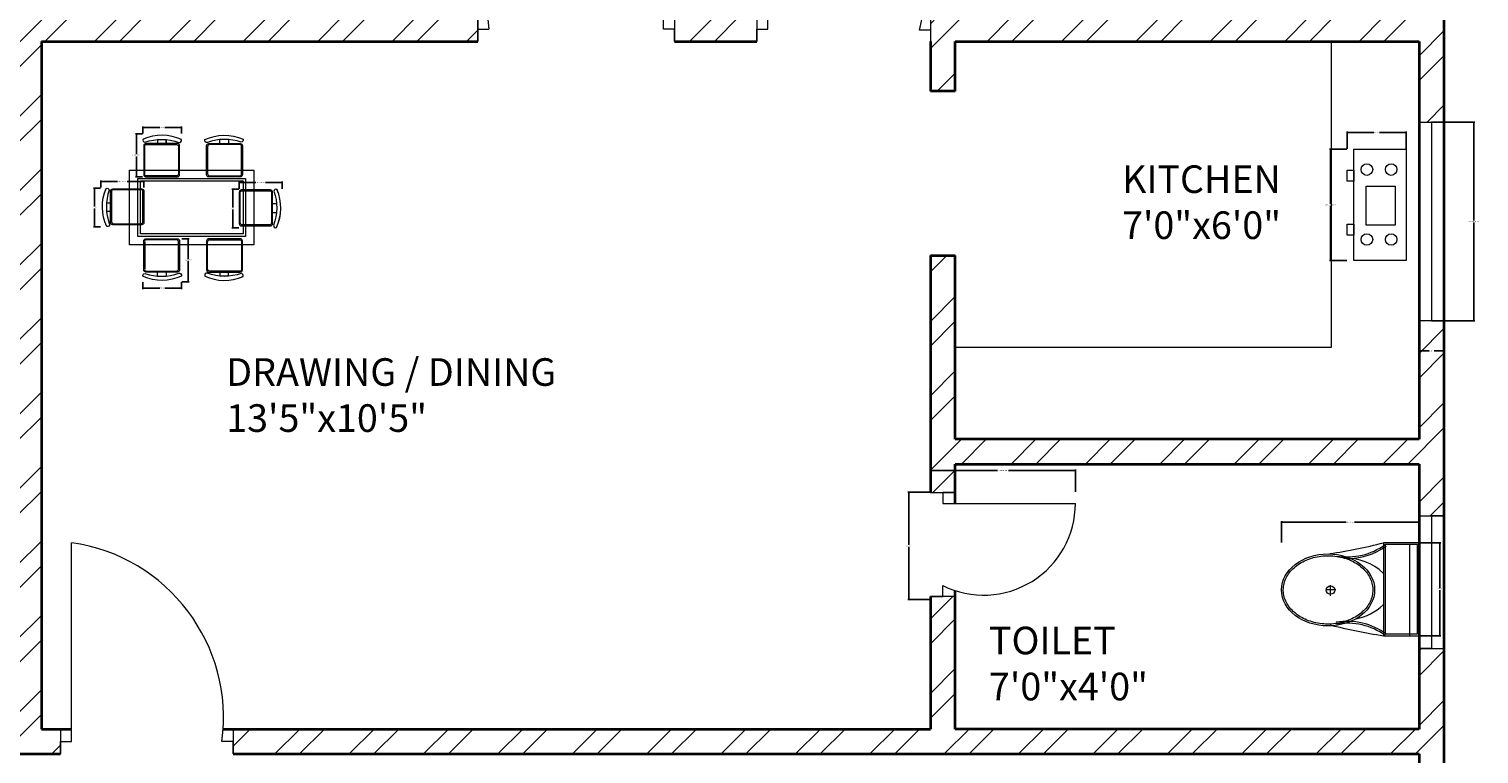
# Model space of a CAD drawing. Units: inches. Extents: x 1944 to 3454, y 1352 to 3055.
# Tile 8 of 17: x 2314 to 2576, y 1900 to 2031. Entities that reach past the tile are written whole.
import ezdxf

# ---------------------------------------------------------------- set-up
doc = ezdxf.new("R2010")
doc.units = ezdxf.units.IN
for name, color, linetype, lineweight in [('A-ANNO-DIMS', 2, 'Continuous', 18), ('A-AREA-IDEN', 7, 'Continuous', 18), ('A-DOOR', 3, 'Continuous', 20), ('A-EQPM', 9, 'Continuous', 18), ('A-FLOR-CASE', 8, 'Continuous', 20), ('A-FLOR-FIXT', 9, 'Continuous', 18), ('A-FURN', 8, 'Continuous', 13), ('A-GLAZ', 4, 'Continuous', 18), ('A-WALL', 7, 'Continuous', 35), ('A-WALL-PATT', 252, 'Continuous', 13)]:
    doc.layers.add(name, color=color, linetype=linetype, lineweight=lineweight)
doc.styles.get("Standard").update_dxf_attribs({"font": 'arial.ttf'})
doc.dimstyles.get("Standard").update_dxf_attribs({"dimtxt": 0.18, "dimasz": 0.18, "dimexe": 0.18, "dimexo": 0.0625, "dimgap": 0.09, "dimtad": 0, "dimtih": 1, "dimtoh": 1, "dimdec": 4, "dimzin": 0, "dimdsep": 46, "dimtxsty": 'Standard', "dimcen": 0.09, "dimadec": 0, "dimazin": 0, "dimtfac": 1, "dimtdec": 4, "dimtofl": 0, "dimtmove": 0, "dimatfit": 3, "dimfxl": 1, "dimtolj": 1, "dimtzin": 0, "dimarcsym": 0})

# ---------------------------------------------------------------- blocks, each defined once
blk = doc.blocks.new('A$C31115884')
for p, q in [((283.1, 497.7), (223.4, 497.7)), ((257.5, 466.4), (257.5, 523.2)), ((0, 200), (0, 0)), ((520, 200), (0, 200)), ((10, 190), (10, 10)), ((510, 190), (10, 190)), ((510, 10), (510, 190)), ((520, 0), (520, 200)), ((510, 54.5), (0, 54.5)), ((10, 10), (510, 10)), ((0, 0), (520, 0))]:
    blk.add_line(p, q)
blk.add_circle((255.6, 496.4), 23.6)
for centre, radius, start, end in [((2777.7, -204.6), 2807, 165.4549, 171.71327), ((3237, 905), 2807, 188.28673, 194.5451), ((-294.5, 403.3), 364.7, 324.20913, 9.34987), ((-294.5, 403.3), 374.7, 324.20913, 9.34987), ((139.5, 406.2), 293.5, 315.84364, 2.65635), ((805.8, 403.3), 374.7, 179.20365, 215.79087), ((805.8, 403.3), 364.7, 170.65013, 215.79087), ((383.6, 406.2), 293.5, 190.27735, 224.15636)]:
    blk.add_arc(centre, radius, start, end)
blk.add_ellipse((256.2, 509.9), major_axis=(0, -260.7), ratio=0.772727)
blk.add_open_spline([(256.2, 259.2), (263.1, 259.2), (270, 259.7), (287.8, 262.3), (298.7, 265.1), (319.9, 273.1), (330.2, 278.4), (350.1, 291.1), (359.7, 298.7), (377.7, 315.9), (386.2, 325.5), (401.7, 346.6), (408.8, 358.1), (421.3, 382.5), (426.8, 395.5), (435.9, 422.4), (439.5, 436.4), (444.8, 465.1), (446.5, 479.7), (447.9, 509.2), (447.6, 524), (445, 553.3), (442.7, 567.8), (436.3, 596), (432.1, 609.7), (421.9, 636), (416, 648.6), (402.5, 672.1), (395, 683), (378.6, 703), (369.8, 712.1), (351.1, 728), (341.3, 734.8), (320.9, 746.2), (310.4, 750.7), (288.9, 757.3), (278, 759.4), (256, 761), (245, 760.6), (223.1, 757.2), (212.3, 754.3), (191.1, 746.1), (180.8, 740.7), (160.9, 727.8), (151.4, 720.1), (133.5, 702.7), (125.1, 693), (109.6, 671.7), (102.6, 660.2), (90.2, 635.7), (84.9, 622.7), (76, 595.6), (72.4, 581.6), (67.2, 552.9), (65.6, 538.2), (64.4, 508.8), (64.8, 494), (67.5, 464.7), (69.9, 450.2), (76.6, 422), (80.8, 408.3), (91.1, 382.2), (97.2, 369.7), (110.8, 346.3), (118.4, 335.4), (134.8, 315.6), (143.7, 306.7), (162.4, 290.9), (172.3, 284.2), (192.8, 273), (203.3, 268.6), (224.8, 262.2), (235.8, 260.2), (249.9, 259.3), (253, 259.2), (256.2, 259.2)], degree=3, knots=[0, 0, 0, 0, 0.110105, 0.110105, 0.285049, 0.285049, 0.459994, 0.459994, 0.634938, 0.634938, 0.809882, 0.809882, 0.984827, 0.984827, 1.159771, 1.159771, 1.334715, 1.334715, 1.50966, 1.50966, 1.684604, 1.684604, 1.859549, 1.859549, 2.034493, 2.034493, 2.209437, 2.209437, 2.384382, 2.384382, 2.559326, 2.559326, 2.73427, 2.73427, 2.909215, 2.909215, 3.084159, 3.084159, 3.259103, 3.259103, 3.434048, 3.434048, 3.608992, 3.608992, 3.783936, 3.783936, 3.958881, 3.958881, 4.133825, 4.133825, 4.30877, 4.30877, 4.483714, 4.483714, 4.658658, 4.658658, 4.833603, 4.833603, 5.008547, 5.008547, 5.183491, 5.183491, 5.358436, 5.358436, 5.53338, 5.53338, 5.708324, 5.708324, 5.883269, 5.883269, 6.058213, 6.058213, 6.233158, 6.233158, 6.283185, 6.283185, 6.283185, 6.283185])
blk = doc.blocks.new('COOKTOP-4B-01')
for points in [[(0, 20.18), (9.48, 20.18), (9.48, 0), (0, 0)], [(2, 13.79), (7.26, 13.79), (7.26, 6.73), (2, 6.73)], [(9.48, 15.59), (10.71, 15.59), (10.71, 13.59), (9.48, 13.59)], [(9.48, 5.81), (10.71, 5.81), (10.71, 3.8), (9.48, 3.8)]]:
    blk.add_lwpolyline(points, close=True)
for centre in [(2.74, 16.38), (7.14, 16.38), (2.74, 3.71), (7.14, 3.71)]:
    blk.add_circle(centre, 1.05)
blk = doc.blocks.new('DOOR-SWING-36IN-01')
for p, q in [((33.61, 2.25), (33.61, 38.25)), ((0, 4.5), (0, 0)), ((0, 0), (0, 4.5)), ((0, 4.5), (0, 2.25)), ((35.61, 4.5), (35.61, 0)), ((0, 2.25), (2, 2.25)), ((35.61, 2.25), (33.61, 2.25)), ((35.61, 0), (35.61, 2.25))]:
    blk.add_line(p, q)
blk.add_arc((33.61, 6.37), 31.88, 90, 187.4328)
blk = doc.blocks.new('DOOR-SWING-36IN-02')
for p, q in [((2, 2.65), (2, 38.65)), ((0, 4.9), (0, 0.4)), ((0, 0.4), (0, 2.65)), ((0, 2.65), (2, 2.65)), ((31.45, 4.9), (31.45, 0)), ((31.45, 2.45), (29.45, 2.45))]:
    blk.add_line(p, q)
blk.add_arc((2, 10.14), 28.51, 344.3464, 90)
blk = doc.blocks.new('DOOR-SWING-24IN-05')
for p, q in [((0, 18.87), (4.5, 18.87)), ((4.5, 18.87), (2.25, 18.87)), ((2.25, 18.87), (2.25, 16.87)), ((2.25, 16.87), (26.25, 16.87)), ((4.5, 0), (0, 0)), ((0, 0), (2.25, 0)), ((2.25, 0), (2.25, 2))]:
    blk.add_line(p, q)
blk.add_arc((9.64, 16.87), 16.61, 243.5781, 0)
blk = doc.blocks.new('DOOR-SWING-36IN-09')
for p, q in [((2, 2.25), (2, 38.25)), ((0, 4.5), (0, 0)), ((31.24, 4.5), (31.24, 0)), ((0, 0), (0, 2.25)), ((0, 2.25), (2, 2.25)), ((31.24, 2.25), (29.24, 2.25)), ((31.24, 0), (31.24, 2.25))]:
    blk.add_line(p, q)
blk.add_arc((-2.49, 6.55), 32.02, 352.2825, 81.9468)
blk = doc.blocks.new('WINDOW-PLAN-24.00IN-01')
for p, q in [((2.25, 24), (0, 24)), ((0, 24), (4.5, 24)), ((2.25, 0), (2.25, 24)), ((0, 0), (4.5, 0)), ((4.5, 0), (2.25, 0))]:
    blk.add_line(p, q)
blk = doc.blocks.new('WINDOW-PLAN-36.00IN-02')
for p, q in [((0, 36), (4.5, 36)), ((4.5, 36), (2.25, 36)), ((2.25, 36), (2.25, 0)), ((4.5, 0), (0, 0)), ((2.25, 0), (4.5, 0))]:
    blk.add_line(p, q)
blk = doc.blocks.new('TABLE-DINING-01')
for points in [[(0, 13.51), (22.52, 13.51), (22.52, 0), (0, 0)], [(0, 13.51), (22.52, 13.51), (22.52, 0), (0, 0)], [(1.5, 12.01), (21.02, 12.01), (21.02, 1.5), (1.5, 1.5)], [(1.5, 12.01), (21.02, 12.01), (21.02, 1.5), (1.5, 1.5)], [(1.95, 11.56), (20.57, 11.56), (20.57, 1.95), (1.95, 1.95)], [(1.95, 11.56), (20.57, 11.56), (20.57, 1.95), (1.95, 1.95)]]:
    blk.add_lwpolyline(points, close=True)
blk = doc.blocks.new('CHAIR-DINING-03')
for points in [[(6.03, 6.44, 0.414214), (5.63, 6.84), (0.4, 6.84, 0.414214), (0, 6.44), (0, 0.74, 0.414214), (0.4, 0.35), (5.63, 0.35, 0.414214), (6.03, 0.74), (6.03, 6.44)], [(6.28, 6.62, -0.175809), (6.23, 0.48, 0.578392), (6.74, 0.02, 0.214524), (6.84, 6.94, 0.552014), (6.28, 6.62, -0.065079)], [(6.03, 2.74), (6.75, 2.74, -0.064759)]]:
    blk.add_lwpolyline(points, format="xyb")
blk.add_lwpolyline([(5.85, 6.44), (5.85, 0.92, -0.414214), (5.45, 0.52), (0.58, 0.52, -0.414214), (0.18, 0.92), (0.18, 6.44, -0.512069), (0.58, 6.66), (5.45, 6.66, -0.512069)], format="xyb", close=True)
blk.add_lwpolyline([(6.77, 4.34), (6.03, 4.34)])
blk = doc.blocks.new('CHAIR-DINING-05')
for points in [[(6.44, 1.5, 0.414214), (6.84, 1.9), (6.84, 7.13, 0.414214), (6.44, 7.53), (0.74, 7.53, 0.414214), (0.34, 7.13), (0.34, 1.9, 0.414214), (0.74, 1.5), (6.44, 1.5)], [(6.62, 1.25, -0.175809), (0.48, 1.3, 0.578392), (0.02, 0.79, 0.214524), (6.94, 0.7, 0.552014), (6.62, 1.25, -0.065079)], [(2.74, 1.5), (2.74, 0.78, -0.064759)]]:
    blk.add_lwpolyline(points, format="xyb")
blk.add_lwpolyline([(6.44, 1.68), (0.92, 1.68, -0.414214), (0.52, 2.08), (0.52, 6.95, -0.414214), (0.92, 7.35), (6.44, 7.35, -0.512069), (6.66, 6.95), (6.66, 2.08, -0.512069)], format="xyb", close=True)
blk.add_lwpolyline([(4.34, 0.77), (4.34, 1.5)])
blk = doc.blocks.new('CHAIR-DINING-06')
for points in [[(0.37, 6.28, -0.175809), (6.5, 6.23, 0.578392), (6.97, 6.74, 0.214524), (0.04, 6.84, 0.552014), (0.37, 6.28, -0.065079)], [(6.24, 6.03), (0.55, 6.03, 0.414214), (0.15, 5.63), (0.15, 0.4, 0.414214), (0.55, 0), (6.24, 0, 0.414214), (6.64, 0.4), (6.64, 5.63, 0.414214), (6.24, 6.03)], [(4.24, 6.03), (4.24, 6.75, -0.064759)]]:
    blk.add_lwpolyline(points, format="xyb")
blk.add_lwpolyline([(0.55, 5.85), (6.06, 5.85, -0.414214), (6.46, 5.46), (6.46, 0.58, -0.414214), (6.06, 0.18), (0.55, 0.18, -0.512069), (0.33, 0.58), (0.33, 5.46, -0.512069)], format="xyb", close=True)
blk.add_lwpolyline([(2.65, 6.77), (2.65, 6.03)])
blk = doc.blocks.new('CHAIR-DINING-07')
for points in [[(1.3, 0.48, -0.578392), (0.79, 0.02, -0.214524), (0.7, 6.94, -0.552014), (1.25, 6.62, 0.175809), (1.3, 0.48)], [(1.5, 6.44, -0.414214), (1.9, 6.84), (7.13, 6.84, -0.414214), (7.53, 6.44), (7.53, 0.74, -0.414214), (7.13, 0.34), (1.9, 0.34, -0.414214), (1.5, 0.74), (1.5, 6.44)], [(1.5, 2.74), (0.78, 2.74, 0.064759)]]:
    blk.add_lwpolyline(points, format="xyb")
blk.add_lwpolyline([(1.68, 6.44), (1.68, 0.92, 0.414214), (2.08, 0.52), (6.95, 0.52, 0.414214), (7.35, 0.92), (7.35, 6.44, 0.512069), (6.95, 6.66), (2.08, 6.66, 0.512069)], format="xyb", close=True)
blk.add_lwpolyline([(0.77, 4.34), (1.5, 4.34)])
blk = doc.blocks.new('CHAIR-DINING-08')
for points in [[(1.3, 0.48, -0.578392), (0.79, 0.02, -0.214524), (0.7, 6.94, -0.552014), (1.25, 6.62, 0.175809), (1.3, 0.48)], [(1.5, 6.44, -0.414214), (1.9, 6.84), (7.13, 6.84, -0.414214), (7.53, 6.44), (7.53, 0.74, -0.414214), (7.13, 0.35), (1.9, 0.35, -0.414214), (1.5, 0.74), (1.5, 6.44)], [(1.5, 2.74), (0.78, 2.74, 0.064759)]]:
    blk.add_lwpolyline(points, format="xyb")
blk.add_lwpolyline([(1.68, 6.44), (1.68, 0.92, 0.414214), (2.08, 0.52), (6.95, 0.52, 0.414214), (7.35, 0.92), (7.35, 6.44, 0.512069), (6.95, 6.66), (2.08, 6.66, 0.512069)], format="xyb", close=True)
blk.add_lwpolyline([(0.77, 4.34), (1.5, 4.34)])
blk = doc.blocks.new('CHAIR-DINING-09')
for points in [[(6.24, 1.5), (0.55, 1.5, -0.414214), (0.15, 1.9), (0.15, 7.13, -0.414214), (0.55, 7.53), (6.24, 7.53, -0.414214), (6.64, 7.13), (6.64, 1.9, -0.414214), (6.24, 1.5)], [(6.5, 1.3, -0.578392), (6.97, 0.79, -0.214524), (0.04, 0.7, -0.552014), (0.37, 1.25, 0.175809), (6.5, 1.3)], [(4.24, 1.5), (4.24, 0.78, 0.064759)]]:
    blk.add_lwpolyline(points, format="xyb")
blk.add_lwpolyline([(0.55, 1.68), (6.06, 1.68, 0.414214), (6.46, 2.08), (6.46, 6.95, 0.414214), (6.06, 7.35), (0.55, 7.35, 0.512069), (0.33, 6.95), (0.33, 2.08, 0.512069)], format="xyb", close=True)
blk.add_lwpolyline([(2.65, 0.77), (2.65, 1.5)])
blk = doc.blocks.new('*D66')
at = {"layer": 'A-ANNO-DIMS', "color": 0, "lineweight": -2, "transparency": 16777216}
for p, q in [((2540.4, 1938.4), (2540.4, 1942.25)), ((2540.58, 1942.07), (2552.08, 1942.07)), ((2565.14, 1942.07), (2553.64, 1942.07)), ((2565.32, 1938.4), (2565.32, 1942.25))]:
    blk.add_line(p, q, dxfattribs=at)
at = {"layer": 'A-ANNO-DIMS', "color": 0, "transparency": 16777216}
for points in [[(2540.58, 1942.1), (2540.58, 1942.04), (2540.4, 1942.07)], [(2565.14, 1942.1), (2565.14, 1942.04), (2565.32, 1942.07)]]:
    blk.add_solid(points, dxfattribs=at)
at = {"layer": 'Defpoints', "color": 0, "transparency": 16777216}
for p in [(2540.4, 1942.07), (2540.4, 1938.33), (2565.32, 1938.33)]:
    blk.add_point(p, dxfattribs=at)
at = {"layer": 'A-ANNO-DIMS', "color": 0, "transparency": 16777216, "insert": (2552.86, 1942.07), "char_height": 0.18, "attachment_point": 5}
blk.add_mtext('\\A1;WC 25 TYP.', dxfattribs=at)
blk = doc.blocks.new('*D67')
at = {"layer": 'A-ANNO-DIMS', "color": 0, "lineweight": -2, "transparency": 16777216}
for p, q in [((2565.38, 1938.33), (2569.24, 1938.33)), ((2569.06, 1938.15), (2569.06, 1930.1)), ((2569.06, 1921.69), (2569.06, 1929.74)), ((2565.38, 1921.51), (2569.24, 1921.51))]:
    blk.add_line(p, q, dxfattribs=at)
at = {"layer": 'A-ANNO-DIMS', "color": 0, "transparency": 16777216}
for points in [[(2569.03, 1938.15), (2569.09, 1938.15), (2569.06, 1938.33)], [(2569.03, 1921.69), (2569.09, 1921.69), (2569.06, 1921.51)]]:
    blk.add_solid(points, dxfattribs=at)
at = {"layer": 'Defpoints', "color": 0, "transparency": 16777216}
for p in [(2565.32, 1938.33), (2569.06, 1938.33), (2565.32, 1921.51)]:
    blk.add_point(p, dxfattribs=at)
at = {"layer": 'A-ANNO-DIMS', "color": 0, "transparency": 16777216, "insert": (2569.06, 1929.92), "char_height": 0.18, "attachment_point": 5}
blk.add_mtext('\\A1;17 TYP.', dxfattribs=at)
blk = doc.blocks.new('*D68')
at = {"layer": 'A-ANNO-DIMS', "color": 0, "lineweight": -2, "transparency": 16777216}
for p, q in [((2552.23, 2009.61), (2549.09, 2009.61)), ((2549.27, 2009.43), (2549.27, 1999.71)), ((2549.27, 1989.62), (2549.27, 1999.34)), ((2552.23, 1989.44), (2549.09, 1989.44))]:
    blk.add_line(p, q, dxfattribs=at)
at = {"layer": 'A-ANNO-DIMS', "color": 0, "transparency": 16777216}
for points in [[(2549.24, 2009.43), (2549.3, 2009.43), (2549.27, 2009.61)], [(2549.24, 1989.62), (2549.3, 1989.62), (2549.27, 1989.44)]]:
    blk.add_solid(points, dxfattribs=at)
at = {"layer": 'Defpoints', "color": 0, "transparency": 16777216}
for p in [(2552.29, 2009.61), (2549.27, 1989.44), (2552.29, 1989.44)]:
    blk.add_point(p, dxfattribs=at)
at = {"layer": 'A-ANNO-DIMS', "color": 0, "transparency": 16777216, "insert": (2549.27, 1999.53), "char_height": 0.18, "attachment_point": 5}
blk.add_mtext('\\A1;COOKTOP 20 TYP.', dxfattribs=at)
blk = doc.blocks.new('*D69')
at = {"layer": 'A-ANNO-DIMS', "color": 0, "lineweight": -2, "transparency": 16777216}
for p, q in [((2552.29, 2009.68), (2552.29, 2012.82)), ((2552.47, 2012.64), (2557.13, 2012.64)), ((2562.82, 2012.64), (2558.17, 2012.64)), ((2563, 2009.68), (2563, 2012.82))]:
    blk.add_line(p, q, dxfattribs=at)
at = {"layer": 'A-ANNO-DIMS', "color": 0, "transparency": 16777216}
for points in [[(2552.47, 2012.67), (2552.47, 2012.61), (2552.29, 2012.64)], [(2562.82, 2012.67), (2562.82, 2012.61), (2563, 2012.64)]]:
    blk.add_solid(points, dxfattribs=at)
at = {"layer": 'Defpoints', "color": 0, "transparency": 16777216}
for p in [(2552.29, 2012.64), (2552.29, 2009.61), (2563, 2009.61)]:
    blk.add_point(p, dxfattribs=at)
at = {"layer": 'A-ANNO-DIMS', "color": 0, "transparency": 16777216, "insert": (2557.65, 2012.64), "char_height": 0.18, "attachment_point": 5}
blk.add_mtext('\\A1;11 TYP.', dxfattribs=at)
blk = doc.blocks.new('*D72')
at = {"layer": 'A-ANNO-DIMS', "color": 0, "lineweight": -2, "transparency": 16777216}
for p, q in [((2569.88, 2014.5), (2575.4, 2014.5)), ((2575.22, 2014.32), (2575.22, 1996.68)), ((2575.22, 1978.68), (2575.22, 1996.32)), ((2569.88, 1978.5), (2575.4, 1978.5))]:
    blk.add_line(p, q, dxfattribs=at)
at = {"layer": 'A-ANNO-DIMS', "color": 0, "transparency": 16777216}
for points in [[(2575.19, 2014.32), (2575.25, 2014.32), (2575.22, 2014.5)], [(2575.19, 1978.68), (2575.25, 1978.68), (2575.22, 1978.5)]]:
    blk.add_solid(points, dxfattribs=at)
at = {"layer": 'Defpoints', "color": 0, "transparency": 16777216}
for p in [(2569.82, 2014.5), (2575.22, 2014.5), (2569.82, 1978.5)]:
    blk.add_point(p, dxfattribs=at)
at = {"layer": 'A-ANNO-DIMS', "color": 0, "transparency": 16777216, "insert": (2575.22, 1996.5), "char_height": 0.18, "attachment_point": 5}
blk.add_mtext('\\A1;WINDOW 36 TYP.', dxfattribs=at)
blk = doc.blocks.new('*D73')
at = {"layer": 'A-ANNO-DIMS', "color": 0, "lineweight": -2, "transparency": 16777216}
for p, q in [((2565.32, 1978.44), (2565.32, 1972.92)), ((2569.82, 1978.44), (2569.82, 1972.92)), ((2565.5, 1973.1), (2567.11, 1973.1)), ((2569.64, 1973.1), (2568.03, 1973.1))]:
    blk.add_line(p, q, dxfattribs=at)
at = {"layer": 'A-ANNO-DIMS', "color": 0, "transparency": 16777216}
for points in [[(2565.5, 1973.13), (2565.5, 1973.07), (2565.32, 1973.1)], [(2569.64, 1973.13), (2569.64, 1973.07), (2569.82, 1973.1)]]:
    blk.add_solid(points, dxfattribs=at)
at = {"layer": 'Defpoints', "color": 0, "transparency": 16777216}
for p in [(2565.32, 1978.5), (2569.82, 1978.5), (2569.82, 1973.1)]:
    blk.add_point(p, dxfattribs=at)
at = {"layer": 'A-ANNO-DIMS', "color": 0, "transparency": 16777216, "insert": (2567.57, 1973.1), "char_height": 0.18, "attachment_point": 5}
blk.add_mtext('\\A1;5 TYP.', dxfattribs=at)
blk = doc.blocks.new('*D124')
at = {"layer": 'A-ANNO-DIMS', "color": 0, "lineweight": -2, "transparency": 16777216}
for p, q in [((2476.82, 1947.53), (2476.82, 1951.59)), ((2477, 1951.41), (2488.96, 1951.41)), ((2502.89, 1951.41), (2490.94, 1951.41)), ((2503.07, 1947.53), (2503.07, 1951.59))]:
    blk.add_line(p, q, dxfattribs=at)
at = {"layer": 'A-ANNO-DIMS', "color": 0, "transparency": 16777216}
for points in [[(2477, 1951.44), (2477, 1951.38), (2476.82, 1951.41)], [(2502.89, 1951.44), (2502.89, 1951.38), (2503.07, 1951.41)]]:
    blk.add_solid(points, dxfattribs=at)
at = {"layer": 'Defpoints', "color": 0, "transparency": 16777216}
for p in [(2503.07, 1951.41), (2476.82, 1947.47), (2503.07, 1947.47)]:
    blk.add_point(p, dxfattribs=at)
at = {"layer": 'A-ANNO-DIMS', "color": 0, "transparency": 16777216, "insert": (2489.95, 1951.41), "char_height": 0.18, "attachment_point": 5}
blk.add_mtext('\\A1;SWING 26 TYP.', dxfattribs=at)
blk = doc.blocks.new('*D125')
at = {"layer": 'A-ANNO-DIMS', "color": 0, "lineweight": -2, "transparency": 16777216}
for p, q in [((2476.76, 1947.47), (2472.7, 1947.47)), ((2472.88, 1947.29), (2472.88, 1937.94)), ((2472.88, 1928.22), (2472.88, 1937.57)), ((2476.76, 1928.04), (2472.7, 1928.04))]:
    blk.add_line(p, q, dxfattribs=at)
at = {"layer": 'A-ANNO-DIMS', "color": 0, "transparency": 16777216}
for points in [[(2472.85, 1947.29), (2472.91, 1947.29), (2472.88, 1947.47)], [(2472.85, 1928.22), (2472.91, 1928.22), (2472.88, 1928.04)]]:
    blk.add_solid(points, dxfattribs=at)
at = {"layer": 'Defpoints', "color": 0, "transparency": 16777216}
for p in [(2472.88, 1947.47), (2476.82, 1947.47), (2476.82, 1928.04)]:
    blk.add_point(p, dxfattribs=at)
at = {"layer": 'A-ANNO-DIMS', "color": 0, "transparency": 16777216, "insert": (2472.88, 1937.75), "char_height": 0.18, "attachment_point": 5}
blk.add_mtext('\\A1;19 TYP.', dxfattribs=at)
blk = doc.blocks.new('*D144')
at = {"layer": 'A-ANNO-DIMS', "color": 0, "lineweight": -2, "transparency": 16777216}
for p, q in [((2351.64, 2002.43), (2351.64, 2003.72)), ((2359.44, 2002.43), (2359.44, 2003.72)), ((2351.82, 2003.54), (2354.66, 2003.54)), ((2359.26, 2003.54), (2356.43, 2003.54))]:
    blk.add_line(p, q, dxfattribs=at)
at = {"layer": 'A-ANNO-DIMS', "color": 0, "transparency": 16777216}
for points in [[(2351.82, 2003.57), (2351.82, 2003.51), (2351.64, 2003.54)], [(2359.26, 2003.57), (2359.26, 2003.51), (2359.44, 2003.54)]]:
    blk.add_solid(points, dxfattribs=at)
at = {"layer": 'Defpoints', "color": 0, "transparency": 16777216}
for p in [(2351.64, 2002.37), (2359.44, 2003.54), (2359.44, 2002.37)]:
    blk.add_point(p, dxfattribs=at)
at = {"layer": 'A-ANNO-DIMS', "color": 0, "transparency": 16777216, "insert": (2355.54, 2003.54), "char_height": 0.18, "attachment_point": 5}
blk.add_mtext('\\A1;CHAIR 8 TYP.', dxfattribs=at)
blk = doc.blocks.new('*D145')
at = {"layer": 'A-ANNO-DIMS', "color": 0, "lineweight": -2, "transparency": 16777216}
for p, q in [((2351.58, 2002.37), (2350.29, 2002.37)), ((2350.47, 2002.19), (2350.47, 1999.03)), ((2350.47, 1995.52), (2350.47, 1998.67)), ((2351.58, 1995.34), (2350.29, 1995.34))]:
    blk.add_line(p, q, dxfattribs=at)
at = {"layer": 'A-ANNO-DIMS', "color": 0, "transparency": 16777216}
for points in [[(2350.44, 2002.19), (2350.5, 2002.19), (2350.47, 2002.37)], [(2350.44, 1995.52), (2350.5, 1995.52), (2350.47, 1995.34)]]:
    blk.add_solid(points, dxfattribs=at)
at = {"layer": 'Defpoints', "color": 0, "transparency": 16777216}
for p in [(2350.47, 2002.37), (2351.64, 2002.37), (2351.64, 1995.34)]:
    blk.add_point(p, dxfattribs=at)
at = {"layer": 'A-ANNO-DIMS', "color": 0, "transparency": 16777216, "insert": (2350.47, 1998.85), "char_height": 0.18, "attachment_point": 5}
blk.add_mtext('\\A1;7 TYP.', dxfattribs=at)
blk = doc.blocks.new('*D150')
at = {"layer": 'A-ANNO-DIMS', "color": 0, "lineweight": -2, "transparency": 16777216}
for p, q in [((2334.12, 2012.37), (2332.83, 2012.37)), ((2333.01, 2012.19), (2333.01, 2008.66)), ((2333.01, 2004.76), (2333.01, 2008.29)), ((2334.12, 2004.58), (2332.83, 2004.58))]:
    blk.add_line(p, q, dxfattribs=at)
at = {"layer": 'A-ANNO-DIMS', "color": 0, "transparency": 16777216}
for points in [[(2332.98, 2012.19), (2333.04, 2012.19), (2333.01, 2012.37)], [(2332.98, 2004.76), (2333.04, 2004.76), (2333.01, 2004.58)]]:
    blk.add_solid(points, dxfattribs=at)
at = {"layer": 'Defpoints', "color": 0, "transparency": 16777216}
for p in [(2333.01, 2012.37), (2334.18, 2012.37), (2334.18, 2004.58)]:
    blk.add_point(p, dxfattribs=at)
at = {"layer": 'A-ANNO-DIMS', "color": 0, "transparency": 16777216, "insert": (2333.01, 2008.48), "char_height": 0.18, "attachment_point": 5}
blk.add_mtext('\\A1;CHAIR 8 TYP.', dxfattribs=at)
blk = doc.blocks.new('*D151')
at = {"layer": 'A-ANNO-DIMS', "color": 0, "lineweight": -2, "transparency": 16777216}
for p, q in [((2334.18, 2012.44), (2334.18, 2013.72)), ((2334.36, 2013.54), (2337.24, 2013.54)), ((2341.03, 2013.54), (2338.16, 2013.54)), ((2341.21, 2012.44), (2341.21, 2013.72))]:
    blk.add_line(p, q, dxfattribs=at)
at = {"layer": 'A-ANNO-DIMS', "color": 0, "transparency": 16777216}
for points in [[(2334.36, 2013.57), (2334.36, 2013.51), (2334.18, 2013.54)], [(2341.03, 2013.57), (2341.03, 2013.51), (2341.21, 2013.54)]]:
    blk.add_solid(points, dxfattribs=at)
at = {"layer": 'Defpoints', "color": 0, "transparency": 16777216}
for p in [(2334.18, 2012.37), (2341.21, 2013.54), (2341.21, 2012.37)]:
    blk.add_point(p, dxfattribs=at)
at = {"layer": 'A-ANNO-DIMS', "color": 0, "transparency": 16777216, "insert": (2337.7, 2013.54), "char_height": 0.18, "attachment_point": 5}
blk.add_mtext('\\A1;7 TYP.', dxfattribs=at)
blk = doc.blocks.new('*D154')
at = {"layer": 'A-ANNO-DIMS', "color": 0, "lineweight": -2, "transparency": 16777216}
for p, q in [((2326.59, 2002.63), (2326.59, 2003.91)), ((2326.77, 2003.73), (2329.6, 2003.73)), ((2334.21, 2003.73), (2331.37, 2003.73)), ((2334.39, 2002.63), (2334.39, 2003.91))]:
    blk.add_line(p, q, dxfattribs=at)
at = {"layer": 'A-ANNO-DIMS', "color": 0, "transparency": 16777216}
for points in [[(2326.77, 2003.76), (2326.77, 2003.7), (2326.59, 2003.73)], [(2334.21, 2003.76), (2334.21, 2003.7), (2334.39, 2003.73)]]:
    blk.add_solid(points, dxfattribs=at)
at = {"layer": 'Defpoints', "color": 0, "transparency": 16777216}
for p in [(2334.39, 2003.73), (2326.59, 2002.56), (2334.39, 2002.56)]:
    blk.add_point(p, dxfattribs=at)
at = {"layer": 'A-ANNO-DIMS', "color": 0, "transparency": 16777216, "insert": (2330.49, 2003.73), "char_height": 0.18, "attachment_point": 5}
blk.add_mtext('\\A1;CHAIR 8 TYP.', dxfattribs=at)
blk = doc.blocks.new('*D155')
at = {"layer": 'A-ANNO-DIMS', "color": 0, "lineweight": -2, "transparency": 16777216}
for p, q in [((2326.53, 2002.56), (2325.24, 2002.56)), ((2325.42, 2002.38), (2325.42, 1999.23)), ((2325.42, 1995.72), (2325.42, 1998.87)), ((2326.53, 1995.54), (2325.24, 1995.54))]:
    blk.add_line(p, q, dxfattribs=at)
at = {"layer": 'A-ANNO-DIMS', "color": 0, "transparency": 16777216}
for points in [[(2325.39, 2002.38), (2325.45, 2002.38), (2325.42, 2002.56)], [(2325.39, 1995.72), (2325.45, 1995.72), (2325.42, 1995.54)]]:
    blk.add_solid(points, dxfattribs=at)
at = {"layer": 'Defpoints', "color": 0, "transparency": 16777216}
for p in [(2325.42, 2002.56), (2326.59, 2002.56), (2326.59, 1995.54)]:
    blk.add_point(p, dxfattribs=at)
at = {"layer": 'A-ANNO-DIMS', "color": 0, "transparency": 16777216, "insert": (2325.42, 1999.05), "char_height": 0.18, "attachment_point": 5}
blk.add_mtext('\\A1;7 TYP.', dxfattribs=at)
blk = doc.blocks.new('*D156')
at = {"layer": 'A-ANNO-DIMS', "color": 0, "lineweight": -2, "transparency": 16777216}
for p, q in [((2341.27, 1993.37), (2342.56, 1993.37)), ((2342.38, 1993.19), (2342.38, 1989.65)), ((2342.38, 1985.75), (2342.38, 1989.29)), ((2341.27, 1985.57), (2342.56, 1985.57))]:
    blk.add_line(p, q, dxfattribs=at)
at = {"layer": 'A-ANNO-DIMS', "color": 0, "transparency": 16777216}
for points in [[(2342.35, 1993.19), (2342.41, 1993.19), (2342.38, 1993.37)], [(2342.35, 1985.75), (2342.41, 1985.75), (2342.38, 1985.57)]]:
    blk.add_solid(points, dxfattribs=at)
at = {"layer": 'Defpoints', "color": 0, "transparency": 16777216}
for p in [(2341.21, 1993.37), (2342.38, 1993.37), (2341.21, 1985.57)]:
    blk.add_point(p, dxfattribs=at)
at = {"layer": 'A-ANNO-DIMS', "color": 0, "transparency": 16777216, "insert": (2342.38, 1989.47), "char_height": 0.18, "attachment_point": 5}
blk.add_mtext('\\A1;CHAIR 8 TYP.', dxfattribs=at)
blk = doc.blocks.new('*D157')
at = {"layer": 'A-ANNO-DIMS', "color": 0, "lineweight": -2, "transparency": 16777216}
for p, q in [((2334.18, 1985.51), (2334.18, 1984.22)), ((2341.21, 1985.51), (2341.21, 1984.22)), ((2334.36, 1984.4), (2337.24, 1984.4)), ((2341.03, 1984.4), (2338.16, 1984.4))]:
    blk.add_line(p, q, dxfattribs=at)
at = {"layer": 'A-ANNO-DIMS', "color": 0, "transparency": 16777216}
for points in [[(2334.36, 1984.43), (2334.36, 1984.37), (2334.18, 1984.4)], [(2341.03, 1984.43), (2341.03, 1984.37), (2341.21, 1984.4)]]:
    blk.add_solid(points, dxfattribs=at)
at = {"layer": 'Defpoints', "color": 0, "transparency": 16777216}
for p in [(2334.18, 1985.57), (2341.21, 1985.57), (2341.21, 1984.4)]:
    blk.add_point(p, dxfattribs=at)
at = {"layer": 'A-ANNO-DIMS', "color": 0, "transparency": 16777216, "insert": (2337.7, 1984.4), "char_height": 0.18, "attachment_point": 5}
blk.add_mtext('\\A1;7 TYP.', dxfattribs=at)

msp = doc.modelspace()

# ---------------------------------------------------------------- hatches: boundary and pattern name
at = {"layer": 'A-WALL-PATT'}
h = msp.add_hatch(dxfattribs=at)
h.set_pattern_fill('ANSI32', color=256)
h.paths.add_polyline_path([(2061.822, 2177.596), (2158.181, 2177.596), (2158.181, 2179.846), (2158.181, 2182.096), (2057.322, 2182.096), (2057.322, 2123.452), (2061.822, 2123.452)])
h.paths.add_polyline_path([(2258.993, 2179.846), (2258.993, 2182.096), (2218.838, 2182.096), (2218.838, 2177.596), (2258.993, 2177.596)])
h.paths.add_polyline_path([(2315.822, 2177.596), (2322.722, 2177.596), (2322.722, 2182.096), (2303.186, 2182.096), (2303.186, 2177.596), (2311.322, 2177.596), (2311.322, 2033.596), (2231.355, 2033.596), (2231.355, 2029.096), (2311.322, 2029.096), (2311.322, 1904.596), (2307.941, 1904.596), (2307.941, 1900.096), (2319.277, 1900.096), (2319.277, 1902.346), (2319.277, 1904.596), (2315.822, 1904.596), (2315.822, 2029.096), (2394.855, 2029.096), (2394.855, 2033.596), (2315.822, 2033.596)])
h.paths.add_polyline_path([(2407.334, 2182.096), (2366.1, 2182.096), (2366.1, 2177.596), (2407.334, 2177.596), (2407.334, 2179.846)])
h.paths.add_polyline_path([(2440.322, 2177.596), (2443.866, 2177.596), (2443.866, 2182.096), (2431.827, 2182.096), (2431.827, 2179.846), (2431.827, 2177.596), (2435.822, 2177.596), (2435.822, 2033.596), (2430.464, 2033.596), (2430.464, 2029.096), (2445.372, 2029.096), (2445.372, 2031.346), (2445.372, 2033.596), (2440.322, 2033.596)])
h.paths.add_polyline_path([(2569.822, 2182.096), (2466.481, 2182.096), (2466.481, 2177.596), (2565.322, 2177.596), (2565.322, 2123.452), (2569.822, 2123.452)])
h.paths.add_polyline_path([(2569.822, 2063.452), (2567.572, 2063.452), (2565.322, 2063.452), (2565.322, 2033.596), (2478.08, 2033.596), (2476.822, 2033.596), (2476.822, 2028.698), (2476.822, 2020.069), (2481.322, 2020.069), (2481.322, 2029.096), (2565.322, 2029.096), (2565.322, 2014.5), (2569.822, 2014.5)])
h.paths.add_polyline_path([(2569.822, 1978.5), (2565.322, 1978.5), (2565.322, 1957.096), (2481.322, 1957.096), (2481.322, 1990.369), (2476.822, 1990.369), (2476.822, 1957.096), (2476.822, 1952.596), (2476.822, 1947.471), (2481.322, 1947.471), (2481.322, 1952.596), (2565.322, 1952.596), (2565.322, 1943.2), (2569.822, 1943.2)])
h.paths.add_polyline_path([(2569.822, 1919.2), (2565.322, 1919.2), (2565.322, 1904.596), (2481.322, 1904.596), (2481.322, 1928.596), (2476.822, 1928.596), (2476.822, 1904.596), (2350.518, 1904.596), (2350.518, 1900.096), (2476.822, 1900.096), (2565.322, 1900.096), (2565.322, 1895.596), (2565.322, 1887.047), (2569.822, 1887.047)])
h.paths.add_polyline_path([(2280.492, 1904.596), (2150.322, 1904.596), (2150.322, 1926.68), (2148.072, 1926.68), (2145.822, 1926.68), (2145.822, 1904.596), (2061.822, 1904.596), (2061.822, 1914.977), (2059.572, 1914.977), (2057.322, 1914.977), (2057.322, 1887.362), (2061.822, 1887.362), (2061.822, 1900.096), (2150.322, 1900.096), (2280.492, 1900.096), (2280.492, 1902.346)])
h.paths.add_polyline_path([(2150.322, 1957.096), (2150.322, 1986.22), (2145.822, 1986.22), (2145.822, 1957.096), (2061.822, 1957.096), (2061.822, 1975.678), (2057.322, 1975.678), (2057.322, 1938.977), (2061.822, 1938.977), (2061.822, 1952.596), (2145.822, 1952.596), (2145.822, 1947.985), (2150.322, 1947.985), (2150.322, 1952.596)])
h.paths.add_polyline_path([(2061.822, 2063.452), (2057.322, 2063.452), (2057.322, 2011.678), (2061.822, 2011.678), (2061.822, 2029.096), (2145.288, 2029.096), (2145.822, 2029.096), (2145.822, 2019.118), (2150.322, 2019.118), (2150.322, 2029.096), (2150.322, 2033.596), (2147.022, 2033.596), (2061.822, 2033.596)])
h.paths.add_polyline_path([(2061.822, 1835.596), (2133.822, 1835.596), (2133.822, 1794.415), (2138.322, 1794.415), (2138.322, 1835.596), (2231.726, 1835.596), (2231.726, 1840.096), (2061.822, 1840.096), (2061.822, 1851.362), (2057.322, 1851.362), (2057.322, 1810.528), (2061.822, 1810.528)])
h.paths.add_polyline_path([(2061.822, 1774.528), (2059.572, 1774.528), (2057.322, 1774.528), (2057.322, 1723.746), (2061.822, 1723.746), (2061.822, 1735.096), (2133.822, 1735.096), (2133.822, 1731.415), (2138.322, 1731.415), (2138.322, 1759.737), (2133.822, 1759.737), (2133.822, 1739.596), (2061.822, 1739.596)])
h.paths.add_polyline_path([(2061.822, 1678.596), (2147.597, 1678.596), (2147.597, 1680.846), (2147.597, 1683.096), (2138.322, 1683.096), (2138.322, 1710.66), (2136.072, 1710.66), (2133.822, 1710.66), (2133.822, 1683.096), (2061.822, 1683.096), (2061.822, 1699.746), (2057.322, 1699.746), (2057.322, 1645.751), (2061.822, 1645.751)])
h.paths.add_polyline_path([(2061.822, 1585.751), (2057.322, 1585.751), (2057.322, 1530.096), (2158.703, 1530.096), (2158.703, 1534.596), (2061.822, 1534.596)])
h.paths.add_polyline_path([(2191.322, 1678.596), (2195.889, 1678.596), (2195.889, 1683.096), (2181.763, 1683.096), (2181.763, 1680.846), (2181.763, 1678.596), (2186.822, 1678.596), (2186.822, 1534.596), (2181.354, 1534.596), (2181.354, 1530.096), (2196.54, 1530.096), (2196.54, 1532.346), (2196.54, 1534.596), (2191.322, 1534.596)])
h.paths.add_polyline_path([(2315.822, 1678.596), (2402.014, 1678.596), (2402.014, 1683.096), (2355.822, 1683.096), (2355.822, 1835.596), (2360.838, 1835.596), (2360.838, 1840.096), (2351.322, 1840.096), (2351.322, 1683.096), (2273.322, 1683.096), (2273.322, 1840.096), (2263.134, 1840.096), (2263.134, 1837.846), (2263.134, 1835.596), (2268.822, 1835.596), (2268.822, 1683.096), (2227.793, 1683.096), (2227.793, 1678.596), (2311.322, 1678.596), (2311.322, 1534.596), (2302.384, 1534.596), (2302.384, 1530.096), (2324.521, 1530.096), (2324.521, 1532.346), (2324.521, 1534.596), (2315.822, 1534.596)])
h.paths.add_polyline_path([(2440.322, 1678.596), (2443.656, 1678.596), (2443.656, 1683.096), (2432.614, 1683.096), (2432.614, 1680.846), (2432.614, 1678.596), (2435.822, 1678.596), (2435.822, 1534.596), (2440.322, 1534.596)])
h.paths.add_polyline_path([(2409.913, 1534.596), (2369.033, 1534.596), (2369.033, 1530.096), (2409.913, 1530.096)])
h.paths.add_polyline_path([(2259.529, 1532.346), (2259.529, 1534.596), (2218.889, 1534.596), (2218.889, 1532.346), (2218.889, 1530.096), (2259.529, 1530.096)])
h.paths.add_polyline_path([(2569.822, 1584.389), (2567.572, 1584.389), (2565.322, 1584.389), (2565.322, 1534.596), (2465.892, 1534.596), (2465.892, 1530.096), (2569.822, 1530.096)])
h.paths.add_polyline_path([(2505.567, 1530.096), (2501.067, 1530.096), (2501.067, 1494.096), (2381.067, 1494.096), (2381.067, 1530.096), (2376.567, 1530.096), (2376.567, 1489.596), (2381.067, 1489.596), (2505.567, 1489.596), (2505.567, 1494.096)])
h.paths.add_polyline_path([(2127.673, 1530.096), (2123.173, 1530.096), (2123.173, 1489.596), (2127.673, 1489.596), (2252.173, 1489.596), (2252.173, 1494.096), (2252.173, 1530.096), (2247.673, 1530.096), (2247.673, 1494.096), (2127.673, 1494.096)])
h.paths.add_polyline_path([(2251.167, 2222.596), (2126.667, 2222.596), (2122.167, 2222.596), (2122.167, 2182.096), (2126.667, 2182.096), (2126.667, 2218.096), (2210.667, 2218.096), (2234.667, 2218.096), (2246.667, 2218.096), (2246.667, 2182.096), (2251.167, 2182.096), (2251.167, 2218.096)])
h.paths.add_polyline_path([(2501.916, 2222.596), (2497.416, 2222.596), (2372.916, 2222.596), (2372.916, 2218.096), (2372.916, 2182.096), (2377.416, 2182.096), (2377.416, 2218.096), (2497.416, 2218.096), (2497.416, 2182.096), (2501.916, 2182.096)])
h.paths.add_polyline_path([(2569.822, 1700.442), (2565.322, 1700.442), (2565.322, 1683.096), (2493.322, 1683.096), (2493.322, 1709.096), (2488.822, 1709.096), (2488.822, 1683.096), (2475.416, 1683.096), (2475.416, 1680.846), (2475.416, 1678.596), (2488.822, 1678.596), (2565.322, 1678.596), (2565.322, 1644.389), (2569.822, 1644.389)])
h.paths.add_polyline_path([(2569.822, 1773.506), (2565.322, 1773.506), (2565.322, 1739.596), (2493.322, 1739.596), (2493.322, 1754.002), (2488.822, 1754.002), (2488.822, 1729.846), (2491.072, 1729.846), (2493.322, 1729.846), (2493.322, 1735.096), (2565.322, 1735.096), (2565.322, 1724.442), (2569.822, 1724.442)])
h.paths.add_polyline_path([(2569.822, 1851.047), (2567.572, 1851.047), (2565.322, 1851.047), (2565.322, 1840.096), (2395.039, 1840.096), (2395.039, 1837.846), (2395.039, 1835.596), (2488.822, 1835.596), (2488.822, 1798.423), (2493.322, 1798.423), (2493.322, 1835.596), (2565.322, 1835.596), (2565.322, 1809.506), (2569.822, 1809.506)])
h.paths.add_polyline_path([(2347.275, 1955.576), (2414.024, 1955.576), (2414.024, 1974.234), (2347.275, 1974.234)], flags=9)
h.paths.add_polyline_path([(2509.756, 1990.497), (2542.915, 1990.497), (2542.915, 2009.154), (2509.756, 2009.154)], flags=9)

# ---------------------------------------------------------------- linework, layer by layer
at = {"layer": 'A-FLOR-CASE'}
for p, q in [((2549.453, 1973.733), (2549.453, 2029.096)), ((2481.322, 1973.733), (2549.453, 1973.733))]:
    msp.add_line(p, q, dxfattribs=at)
at = {"layer": 'A-FURN'}
for points in [[(2334.57, 2010.856, -0.1758092), (2340.704, 2010.81, 0.5783921), (2341.169, 2011.32, 0.2145244), (2334.245, 2011.413, 0.552014), (2334.57, 2010.856, -0.065079)], [(2345.868, 2010.81, -0.5783921), (2345.403, 2011.321, -0.2145244), (2352.327, 2011.414, -0.552014), (2352.002, 2010.856, 0.1758092), (2345.868, 2010.81)], [(2345.868, 2010.81, -0.5783921), (2345.403, 2011.32, -0.2145244), (2352.327, 2011.413, -0.552014), (2352.002, 2010.856, 0.1758092), (2345.868, 2010.81)], [(2340.444, 2010.61), (2334.749, 2010.61, 0.4142136), (2334.351, 2010.211), (2334.351, 2004.975, 0.4142136), (2334.749, 2004.577), (2340.444, 2004.577, 0.4142136), (2340.842, 2004.975), (2340.842, 2010.211, 0.4142136), (2340.444, 2010.61)], [(2338.444, 2010.61), (2338.444, 2011.33, -0.0647586)], [(2351.823, 2010.61, -0.4142136), (2352.221, 2010.212), (2352.221, 2004.976, -0.4142136), (2351.823, 2004.577), (2346.128, 2004.577, -0.4142136), (2345.73, 2004.976), (2345.73, 2010.212, -0.4142136), (2346.128, 2010.61), (2351.823, 2010.61)], [(2351.823, 2010.61, -0.4142136), (2352.221, 2010.211), (2352.221, 2004.975, -0.4142136), (2351.823, 2004.577), (2346.128, 2004.577, -0.4142136), (2345.73, 2004.975), (2345.73, 2010.211, -0.4142136), (2346.128, 2010.61), (2351.823, 2010.61)], [(2348.128, 2010.61), (2348.128, 2011.33, 0.0647586)], [(2348.128, 2010.61), (2348.128, 2011.33, 0.0647586)], [(2357.677, 2001.804, 0.4142136), (2357.278, 2002.202), (2352.042, 2002.202, 0.4142136), (2351.644, 2001.804), (2351.644, 1996.109, 0.4142136), (2352.042, 1995.711), (2357.278, 1995.711, 0.4142136), (2357.677, 1996.109), (2357.677, 2001.804)], [(2357.923, 2001.983, -0.1758092), (2357.876, 1995.849, 0.5783921), (2358.387, 1995.384, 0.2145244), (2358.48, 2002.308, 0.552014), (2357.923, 2001.983, -0.065079)], [(2357.677, 1998.109), (2358.397, 1998.109, -0.0647586)], [(2351.823, 1987.335, 0.4142136), (2352.221, 1987.733), (2352.221, 1992.969, 0.4142136), (2351.823, 1993.368), (2346.128, 1993.368, 0.4142136), (2345.73, 1992.969), (2345.73, 1987.733, 0.4142136), (2346.128, 1987.335), (2351.823, 1987.335)], [(2352.002, 1987.089, -0.1758093), (2345.868, 1987.135, 0.5783921), (2345.403, 1986.624, 0.2145244), (2352.327, 1986.531, 0.552014), (2352.002, 1987.089, -0.065079)], [(2348.128, 1987.335), (2348.128, 1986.615, -0.0647586)]]:
    msp.add_lwpolyline(points, format="xyb", dxfattribs=at)
for points in [[(2334.752, 2010.43), (2340.264, 2010.43, -0.4142136), (2340.663, 2010.032), (2340.663, 2005.155, -0.4142136), (2340.264, 2004.757), (2334.752, 2004.757, -0.5120695), (2334.531, 2005.155), (2334.531, 2010.032, -0.5120695)], [(2351.82, 2010.431), (2346.308, 2010.431, 0.4142136), (2345.909, 2010.032), (2345.909, 2005.155, 0.4142136), (2346.308, 2004.757), (2351.82, 2004.757, 0.5120695), (2352.042, 2005.155), (2352.042, 2010.032, 0.5120695)], [(2351.82, 2010.43), (2346.308, 2010.43, 0.4142136), (2345.909, 2010.032), (2345.909, 2005.155, 0.4142136), (2346.308, 2004.757), (2351.82, 2004.757, 0.5120695), (2352.042, 2005.155), (2352.042, 2010.032, 0.5120695)], [(2357.497, 2001.801), (2357.497, 1996.289, -0.4142136), (2357.099, 1995.89), (2352.222, 1995.89, -0.4142136), (2351.823, 1996.289), (2351.823, 2001.801, -0.5120695), (2352.222, 2002.022), (2357.099, 2002.022, -0.5120695)], [(2351.82, 1987.514), (2346.308, 1987.514, -0.4142136), (2345.909, 1987.913), (2345.909, 1992.79, -0.4142136), (2346.308, 1993.188), (2351.82, 1993.188, -0.5120695), (2352.042, 1992.79), (2352.042, 1987.913, -0.5120695)]]:
    msp.add_lwpolyline(points, format="xyb", close=True, dxfattribs=at)
for points in [[(2336.85, 2011.343), (2336.85, 2010.61)], [(2349.722, 2011.343), (2349.722, 2010.61)], [(2349.722, 2011.343), (2349.722, 2010.61)], [(2358.41, 1999.703), (2357.677, 1999.703)], [(2349.722, 1986.602), (2349.722, 1987.335)]]:
    msp.add_lwpolyline(points, dxfattribs=at)
at = {"layer": 'A-WALL'}
for p, q in [((2569.822, 2182.096), (2569.822, 1530.096)), ((2315.822, 2029.096), (2315.822, 1904.596)), ((2315.822, 2029.096), (2394.855, 2029.096)), ((2430.464, 2029.096), (2445.372, 2029.096)), ((2476.822, 2029.096), (2476.822, 2020.069)), ((2481.322, 2029.096), (2565.322, 2029.096)), ((2481.322, 2020.069), (2481.322, 2029.096)), ((2565.322, 2029.096), (2565.322, 1957.096)), ((2565.322, 2029.096), (2565.322, 1957.096)), ((2481.322, 2020.069), (2476.822, 2020.069)), ((2476.822, 1990.369), (2481.322, 1990.369)), ((2476.822, 1990.369), (2476.822, 1957.096)), ((2481.322, 1957.096), (2481.322, 1990.369)), ((2476.822, 1957.096), (2476.822, 1952.596)), ((2565.322, 1957.096), (2481.322, 1957.096)), ((2476.822, 1952.596), (2476.822, 1947.471)), ((2481.322, 1952.596), (2565.322, 1952.596)), ((2481.322, 1945.471), (2481.322, 1952.596)), ((2565.322, 1952.596), (2565.322, 1904.596)), ((2565.322, 1952.596), (2565.322, 1904.596)), ((2476.822, 1928.596), (2476.822, 1904.596)), ((2481.322, 1904.596), (2481.322, 1929.677)), ((2315.822, 1904.596), (2321.277, 1904.596)), ((2348.743, 1904.596), (2476.822, 1904.596)), ((2565.322, 1904.596), (2481.322, 1904.596)), ((2307.941, 1900.096), (2319.277, 1900.096)), ((2350.518, 1900.096), (2476.822, 1900.096)), ((2476.822, 1900.096), (2565.322, 1900.096)), ((2565.322, 1900.096), (2565.322, 1840.096)), ((2565.322, 1900.096), (2565.322, 1895.596))]:
    msp.add_line(p, q, dxfattribs=at)

# ---------------------------------------------------------------- block references
at = {"layer": 'A-DOOR'}
for name, p in [('DOOR-SWING-36IN-01', (2394.855, 2029.096)), ('DOOR-SWING-36IN-02', (2445.372, 2028.698)), ('DOOR-SWING-24IN-05', (2476.822, 1928.596)), ('DOOR-SWING-36IN-09', (2319.277, 1900.096))]:
    msp.add_blockref(name, p, dxfattribs=at)
at = {"layer": 'A-EQPM', "rotation": 180}
msp.add_blockref('COOKTOP-4B-01', (2563, 2009.614), dxfattribs=at)
at = {"layer": 'A-FLOR-FIXT', "xscale": 0.0323450304620732, "yscale": 0.0323450304620732, "zscale": 0.0323450304620732, "rotation": 89.99999999999999}
msp.add_blockref('A$C31115884', (2565.322, 1921.514), dxfattribs=at)
at = {"layer": 'A-FURN'}
for name, p in [('CHAIR-DINING-06', (2334.202, 2004.577)), ('TABLE-DINING-01', (2331.785, 1992.288)), ('CHAIR-DINING-07', (2326.853, 1995.561)), ('CHAIR-DINING-08', (2326.853, 1995.56)), ('CHAIR-DINING-03', (2351.644, 1995.365)), ('CHAIR-DINING-09', (2334.202, 1985.835)), ('CHAIR-DINING-09', (2334.202, 1985.835)), ('CHAIR-DINING-05', (2345.385, 1985.835))]:
    msp.add_blockref(name, p, dxfattribs=at)
at = {"layer": 'A-GLAZ'}
msp.add_blockref('WINDOW-PLAN-36.00IN-02', (2565.322, 1978.5), dxfattribs=at)
at = {"layer": 'A-GLAZ', "extrusion": (0, 0, -1), "zscale": -1, "rotation": 180}
msp.add_blockref('WINDOW-PLAN-24.00IN-01', (-2565.322, 1943.2), dxfattribs=at)

# ---------------------------------------------------------------- texts
at = {"layer": 'A-AREA-IDEN', "char_height": 5, "attachment_point": 1}
for s, width, insert in [('KITCHEN\\P7\'0"x6\'0"', 100.95454, (2511.518, 2006.666)), ('DRAWING / DINING\\P13\'5"x10\'5"', 182.48881, (2349.285, 1971.746)), ('TOILET\\P7\'0"x4\'0"', 93.29173, (2487.415, 1923.142))]:
    msp.add_mtext_dynamic_manual_height_columns(s, width=width, gutter_width=12.5, heights=[0], dxfattribs=dict(at, insert=insert))

# ---------------------------------------------------------------- dimensions: what is measured, and where the dimension line sits
at = {"layer": 'A-ANNO-DIMS'}
for base, p1, p2, angle, text, picture, middle in [((2575.222, 2014.5), (2569.822, 1978.5), (2569.822, 2014.5), 90, 'WINDOW <> TYP.', '*D72', (2575.222, 1996.5)), ((2333.015, 2012.374), (2334.184, 2004.577), (2334.184, 2012.374), 90, 'CHAIR <> TYP.', '*D150', (2333.015, 2008.476)), ((2552.292, 2012.641), (2563, 2009.614), (2552.292, 2009.614), 180, '<> TYP.', '*D69', (2557.646, 2012.641)), ((2549.265, 1989.436), (2552.292, 2009.614), (2552.292, 1989.436), 270, 'COOKTOP <> TYP.', '*D68', (2549.265, 1999.525)), ((2325.419, 2002.563), (2326.589, 1995.535), (2326.589, 2002.563), 90, '<> TYP.', '*D155', (2325.419, 1999.049)), ((2350.474, 2002.368), (2351.644, 1995.34), (2351.644, 2002.368), 90, '<> TYP.', '*D145', (2350.474, 1998.854)), ((2342.382, 1993.368), (2341.212, 1985.571), (2341.212, 1993.368), 90, 'CHAIR <> TYP.', '*D156', (2342.382, 1989.469)), ((2472.884, 1947.471), (2476.822, 1928.038), (2476.822, 1947.471), 90, '<> TYP.', '*D125', (2472.884, 1937.754)), ((2540.398, 1942.072), (2565.322, 1938.333), (2540.398, 1938.333), 180, 'WC <> TYP.', '*D66', (2552.86, 1942.072)), ((2569.06, 1938.333), (2565.322, 1921.514), (2565.322, 1938.333), 90, '<> TYP.', '*D67', (2569.06, 1929.923))]:
    dim = msp.add_linear_dim(base=base, p1=p1, p2=p2, angle=angle, text=text, dimstyle='Standard', override={"dimdec": 0, "dimlfac": 1, "dimrnd": 0, "dimzin": 0, "dimdsep": 46, "dimlunit": 2}, dxfattribs=at)
    dim.commit()
    dim.dimension.update_dxf_attribs({"geometry": picture, "text_midpoint": middle})
for base, p1, p2, text, picture, middle in [((2341.212, 2013.544), (2334.184, 2012.374), (2341.212, 2012.374), '<> TYP.', '*D151', (2337.698, 2013.544)), ((2334.386, 2003.733), (2326.589, 2002.563), (2334.386, 2002.563), 'CHAIR <> TYP.', '*D154', (2330.487, 2003.733)), ((2359.441, 2003.538), (2351.644, 2002.368), (2359.441, 2002.368), 'CHAIR <> TYP.', '*D144', (2355.542, 2003.538)), ((2341.212, 1984.401), (2334.184, 1985.571), (2341.212, 1985.571), '<> TYP.', '*D157', (2337.698, 1984.401)), ((2569.821802765, 1973.100264753), (2565.321802765, 1978.500264753), (2569.821802765, 1978.500264753), '<> TYP.', '*D73', (2567.571802765, 1973.100264753)), ((2503.072, 1951.408), (2476.822, 1947.471), (2503.072, 1947.471), 'SWING <> TYP.', '*D124', (2489.947, 1951.408))]:
    dim = msp.add_linear_dim(base=base, p1=p1, p2=p2, text=text, dimstyle='Standard', override={"dimdec": 0, "dimlfac": 1, "dimrnd": 0, "dimzin": 0, "dimdsep": 46, "dimlunit": 2}, dxfattribs=at)
    dim.commit()
    dim.dimension.update_dxf_attribs({"geometry": picture, "text_midpoint": middle})

doc.saveas('drawing.dxf')
